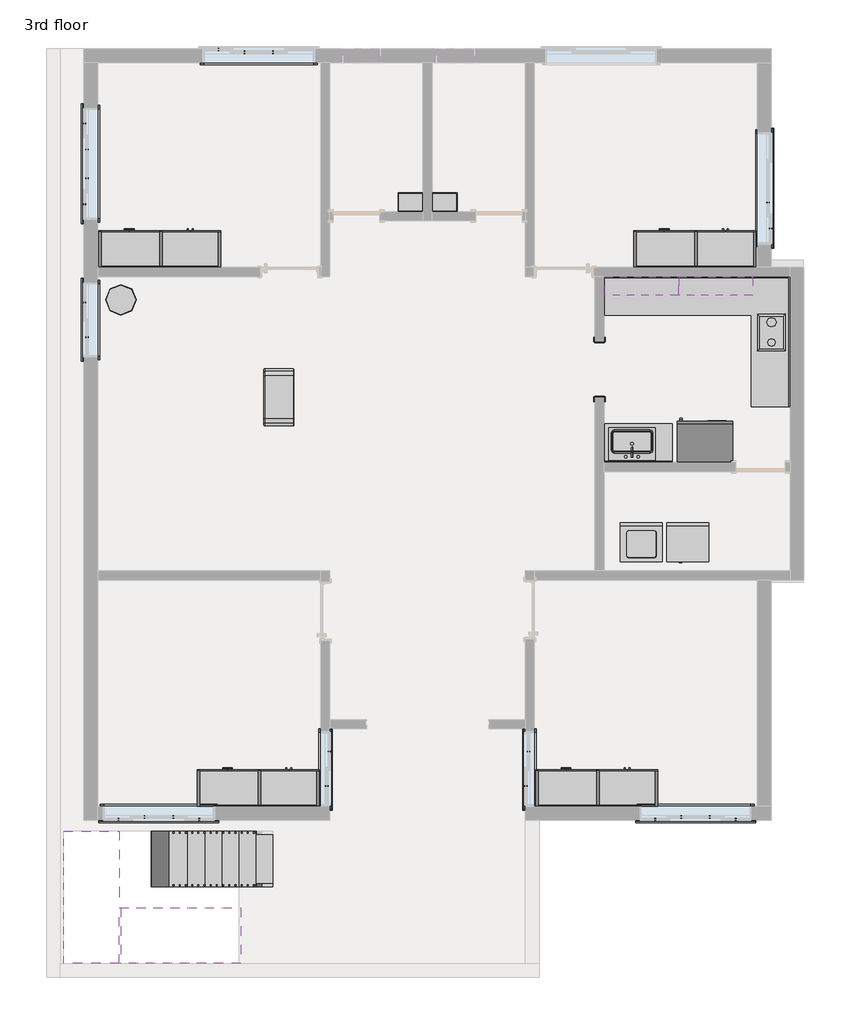
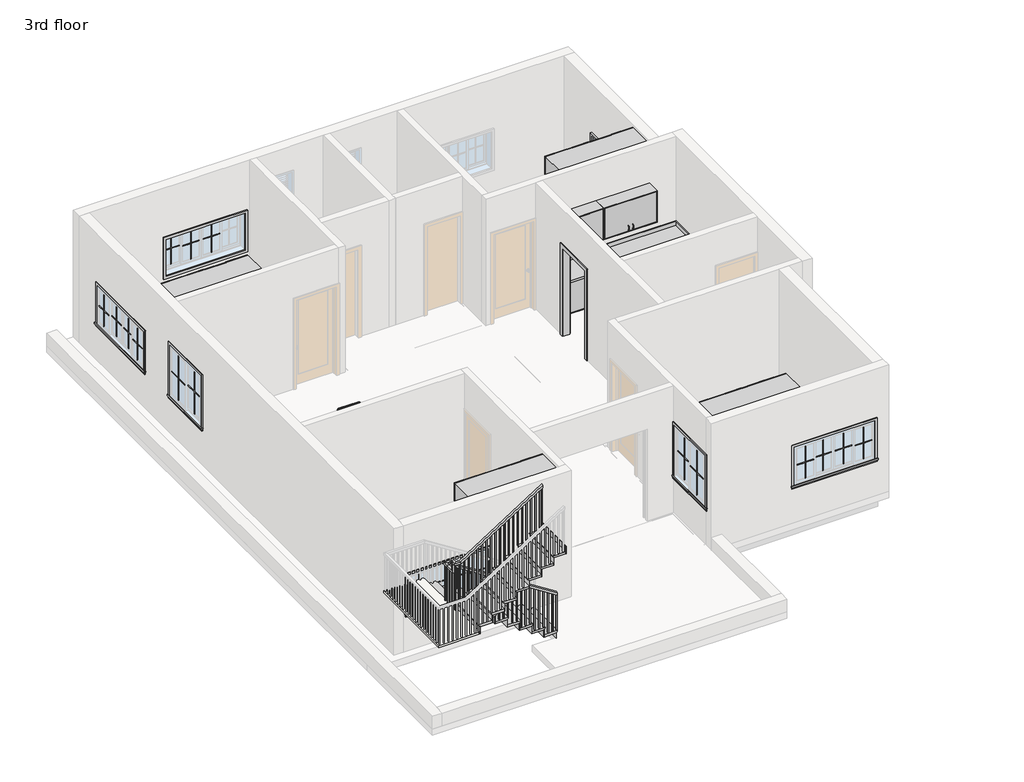
# One storey, part 3 of 4: 42 proxies, 15 furniture elements, 3 flow terminals, 2 stair flights, 1 railing, 1 slab.
# Revit data of these elements (continued)
# Elements 37, 38, 39, 40, 41 (IfcBuildingElementProxy, "Trim-Window-Interior-Flat : Picture Frame")
#   Opening Width = 6' - 0"
#   Opening Height = 3' - 0"
#   Trim Material = Wood - Stained
#   Phase Created = New Construction
#   Materials on its faces: "Wood - Stained"
# Element 42 (IfcBuildingElementProxy, "Washer : 27\" x 25\" x 35\"")
#   Phase Created = New Construction
#   Materials on its faces: "Metal - Paint Finish - Ivory,Matte"
# Element 43 (IfcFlowTerminal, "Sink - Work : 20\"x18\" 2")
#   Mark = "29"
#   Flow Pressure = 8.00 psi
#   Phase Created = New Construction
# Element 44 (IfcFlowTerminal, "Sink - Work : 20\"x18\" 2")
#   Mark = "30"
#   Flow Pressure = 8.00 psi
#   Phase Created = New Construction
# Element 45 (IfcFlowTerminal, "Sink Kitchen-Single : 30\" x 21\"")
#   Mark = "28"
#   Phase Created = New Construction
#   Materials on its faces: "Steel, Polished"
# Element 46 (IfcFurniture)
#   Phase Created = New Construction
# Element 47 (IfcFurniture)
#   Phase Created = New Construction
#   Materials on its faces: "Default", "Default 3", "Default 2"
# Elements 48, 49, 50, 51 (IfcFurniture, "1Wardrobe_6271 : 1Wardrobe_6271")
#   Phase Created = New Construction
#   Materials on its faces: "Phase - Demo", "Default Wall", "Phase - Exist", "Default"
# Element 52 (IfcFurniture, "48\" 2")
#   Phase Created = New Construction
#   Materials on its faces: "Cabinet", "Cabinets - Handles", "Cabinets"
# Element 53 (IfcFurniture, "48\" 3")
#   Phase Created = New Construction
#   Materials on its faces: "Cabinet", "Cabinets - Handles", "Cabinets"
# Element 54 (IfcFurniture, "Base Cabinet-Combo01 : 30\" 2")
#   Phase Created = New Construction
#   Materials on its faces: "Cabinet"
# Element 55 (IfcFurniture, "Base Cabinet-Corner Unit-Square : 36\"")
#   Phase Created = New Construction
#   Materials on its faces: "Cabinets", "Cabinets - Handles"
# Element 56 (IfcFurniture, "Counter Top w Sink Hole : 24\" Depth")
#   Sink Opening Width = 2' - 3"
#   Sink Opening Depth = 1' - 3"
#   Sink Location To Wall = 0' - 6"
#   Sink Location = 2' - 2"
#   Length = 3' - 8"
#   Phase Created = New Construction
#   Materials on its faces: "Counter Top"
# Element 57 (IfcFurniture, "Counter Top-L Shaped : 24\" Depth")
#   Length - Leg 2 = 10' - 0"
#   Length - Leg 1 = 7' - 0"
#   Phase Created = New Construction
#   Materials on its faces: "Counter Top"
# Element 58 (IfcFurniture, "Table-Trio End : 20\" Diameter")
#   Phase Created = New Construction
#   Materials on its faces: "Wood - Birch", "Laminate - Ivory,Matte"
# Elements 59, 60 (IfcFurniture, "Upper Cabinet-Pass-Thru : 48\" x 30\" x 12\"")
#   Phase Created = New Construction
#   Materials on its faces: "Cabinet"
# Element 61 (IfcRailing, "Handrail - Rectangular")
#   Phase Created = New Construction
# Element 62 (IfcSlab, "Non-Monolithic Landing")
#   Phase Created = New Construction
# Elements 63, 64 (IfcStairFlight, "2\" Tread 1\" Nosing 1/4\" Riser")
#   Phase Created = New Construction
# Materials
#   "Metal - Chrome": colour RGB 17 17 17, transparency 0
#   "Metal - Steel, Polished": colour RGB 57 57 57, transparency 0
#   "Metal - Paint Finish - Ivory,Glossy": colour RGB 247 247 239, transparency 0
#   "Door - Frame": colour RGB 118 70 51, transparency 0, Cost = 0
#   "Metal - Paint Finish - Ivory,Matte": colour RGB 247 247 239, transparency 0
#   "Steel, Polished": class "Metal", colour RGB 192 192 192, transparency 0, Description = "Polished steel", Cost = 0
#   "Cabinets - Handles": colour RGB 57 57 57, transparency 0
#   "Cabinets": colour RGB 249 249 249, transparency 0
#   "Wood - Birch": colour RGB 230 196 162, transparency 0
#   "Laminate - Ivory,Matte": colour RGB 127 127 127, transparency 0
#   "Clad - White": class "Wood", colour RGB 242 242 238, transparency 0, Cost = 0
#   "Wood - Stained": class "Wood", colour RGB 224 178 126, transparency 0, Cost = 0
#   "Default": colour RGB 127 127 127, transparency 0, Cost = 0
#   "Default 3": class "Glass", colour RGB 127 127 127, transparency 0
#   "Default 2": class "Plastic", colour RGB 127 127 127, transparency 0
#   "Phase - Demo": class "System", colour RGB 255 0 0, transparency 0.4, Cost = 0
#   "Default Wall": colour RGB 128 128 128, transparency 0, Cost = 0
#   "Phase - Exist": class "System", colour RGB 127 127 127, transparency 0, Cost = 0
#   "Cabinet": colour RGB 204 122 2, transparency 0
#   "Counter Top": class "Wood", colour RGB 226 177 128, transparency 0
